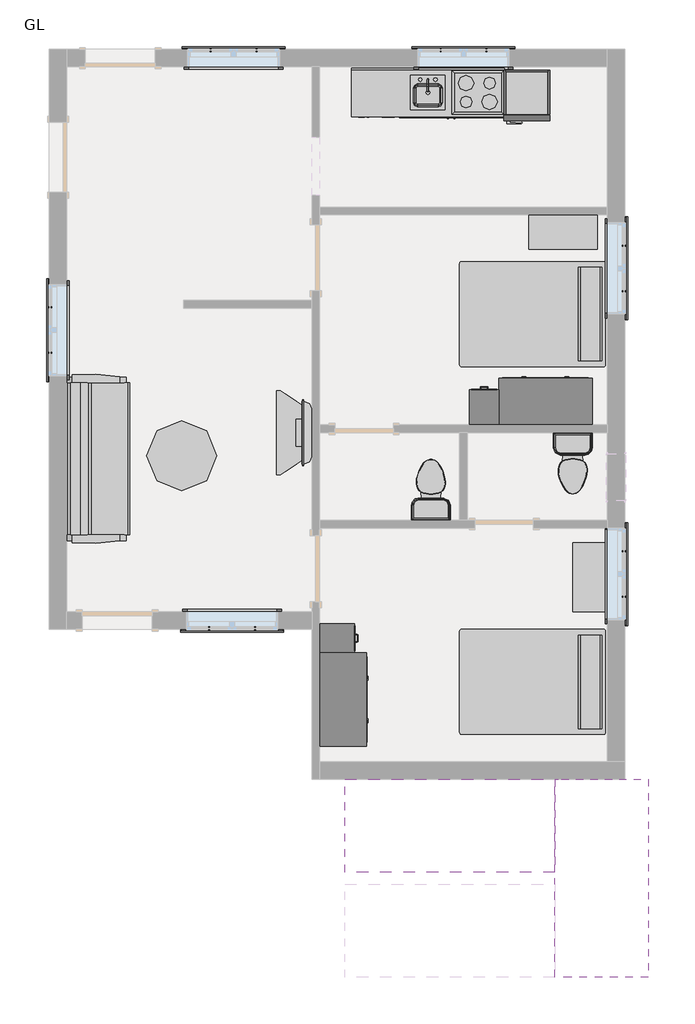
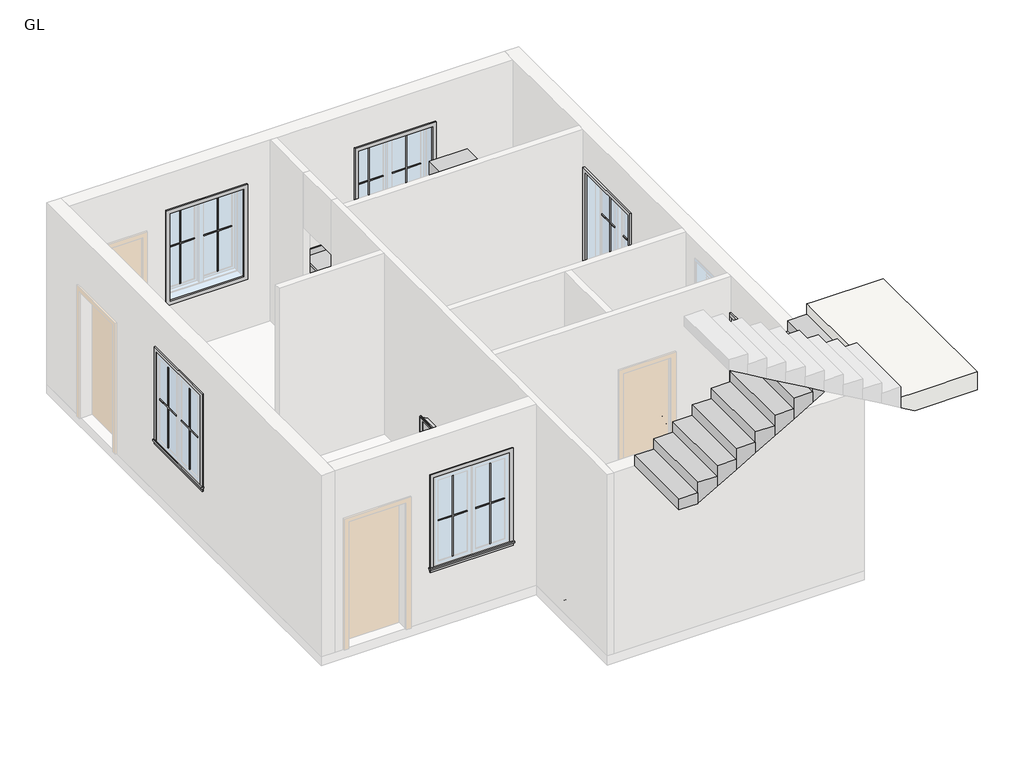
# One storey, part 2 of 2: 28 proxies, 13 furniture elements, 3 flow terminals, 1 slab, 1 stair flight.
"""IFC4 building model written with IfcOpenShell, lengths in millimetres."""

from ifc_helpers import new_model, si_unit, origin, place, context, project, spatial, faceted_brep, transform, mapped, element, save
from components import m_cook_top_4_unit2_0615_x_500mm_c91639ce, m_dishwasher_610_x_610_x_875mm_75336c20, m_kitchenette_medium_m_kitchenette_medium_71e50c56, m_muntin_pattern_2x2_m_muntin_pattern_2x2_d4676b39, m_muntin_pattern_2x2_m_muntin_pattern_2x2_dce6eb8c, m_refrigerator_600_x_660mm_0a899b9c, m_trim_window_exterior_flat_with_sill_a970d7bf, m_trim_window_interior_flat_picture_frame_5bf35ee4, m_sink_kitchen_island_450_x_450mm_f6c2c534, m_toilet_domestic_3d_m_toilet_domestic_3d_ba6479b0, m_toilet_domestic_3d_m_toilet_domestic_3d_1a010dbe, furniture_dc210597, furniture_0810mm_51289c3c, m_bed_standard_1372_x_1905mm_double_64e02cd7, m_cabinet_file_5_drawer_0380_x_0457mm_21dee09a, m_counter_top_w_sink_hole_600mm_depth_2c7d9717, m_dresser_1220_x_1830_x_0610mm_75a9f440, m_furniture_system_storage_cabinet_2_vertical_file_900_x_450_def3fd80, m_sofa_pensi_2134mm_538a523a, m_table_dining_round_0915mm_diameter_394c0b6d

model = new_model("IFC4")

# Units and contexts
model_context = context("Model", 3, world=origin())
ifc_project = project(units=[si_unit("LENGTHUNIT", "METRE", prefix="MILLI")], contexts=[model_context])

# Site, building, storey
site = spatial("IfcSite", under=ifc_project)
building = spatial("IfcBuilding", under=site)
storey = spatial("IfcBuildingStorey", under=building, Name="GL", Elevation=0.0)

# Proxies
placement = place(None, origin())
m_cook_top_4_unit2_0615_x_500mm_shape = m_cook_top_4_unit2_0615_x_500mm_c91639ce(model_context)
element("IfcBuildingElementProxy", 1, Name="M_Cook Top-4 Unit2 : 0615 x 500mm", ObjectType="M_Cook Top-4 Unit2 : 0615 x 500mm", at=placement, inside=storey, context=model_context, shape_type="MappedRepresentation", body=[
    mapped(m_cook_top_4_unit2_0615_x_500mm_shape, transform((1952.0701854, 4546.4851347, 15.0), x_axis=(-1.0, 0.0, 0.0), y_axis=(0.0, -1.0, 0.0), z_axis=(0.0, 0.0, 1.0))),
])
m_dishwasher_610_x_610_x_875mm_shape = m_dishwasher_610_x_610_x_875mm_75336c20(model_context)
element("IfcBuildingElementProxy", 2, Name="M_Dishwasher : 610 x 610 x 875mm", ObjectType="M_Dishwasher : 610 x 610 x 875mm", at=placement, inside=storey, context=model_context, shape_type="MappedRepresentation", body=[
    mapped(m_dishwasher_610_x_610_x_875mm_shape, transform((987.0876539, 4289.8355699, 0.0), x_axis=(-1.0, 0.0, 0.0), y_axis=(0.0, -1.0, 0.0), z_axis=(0.0, 0.0, 1.0))),
])
m_kitchenette_medium_m_kitchenette_medium_shape = m_kitchenette_medium_m_kitchenette_medium_71e50c56(model_context)
element("IfcBuildingElementProxy", 3, Name="M_Kitchenette - Medium : M_Kitchenette - Medium", ObjectType="M_Kitchenette - Medium : M_Kitchenette - Medium", at=placement, inside=storey, context=model_context, shape_type="MappedRepresentation", body=[
    mapped(m_kitchenette_medium_m_kitchenette_medium_shape, transform((1623.3078903, 4861.4851347, 0.0), x_axis=(-1.0, 0.0, 0.0), y_axis=(0.0, -1.0, 0.0), z_axis=(0.0, 0.0, 1.0))),
])
m_muntin_pattern_2x2_m_muntin_pattern_2x2_shape = m_muntin_pattern_2x2_m_muntin_pattern_2x2_d4676b39(model_context)
element("IfcBuildingElementProxy", 4, Name="M_Muntin Pattern_2x2 : M_Muntin Pattern_2x2", ObjectType="M_Muntin Pattern_2x2 : M_Muntin Pattern_2x2", at=placement, inside=storey, context=model_context, shape_type="MappedRepresentation", body=[
    mapped(m_muntin_pattern_2x2_m_muntin_pattern_2x2_shape, transform((1466.9330952, 5099.6101347, 969.85), x_axis=(1.0, 0.0, 0.0), y_axis=(0.0, 1.0, 0.0), z_axis=(0.0, 0.0, 1.0))),
])
element("IfcBuildingElementProxy", 5, Name="M_Muntin Pattern_2x2 : M_Muntin Pattern_2x2", ObjectType="M_Muntin Pattern_2x2 : M_Muntin Pattern_2x2", at=placement, inside=storey, context=model_context, shape_type="MappedRepresentation", body=[
    mapped(m_muntin_pattern_2x2_m_muntin_pattern_2x2_shape, transform((3864.0205952, 2548.5476347, 969.85), x_axis=(0.0, -1.0, 0.0), y_axis=(1.0, 0.0, 0.0), z_axis=(0.0, 0.0, 1.0))),
])
element("IfcBuildingElementProxy", 6, Name="M_Muntin Pattern_2x2 : M_Muntin Pattern_2x2", ObjectType="M_Muntin Pattern_2x2 : M_Muntin Pattern_2x2", at=placement, inside=storey, context=model_context, shape_type="MappedRepresentation", body=[
    mapped(m_muntin_pattern_2x2_m_muntin_pattern_2x2_shape, transform((3864.0205952, -1440.8523653, 969.85), x_axis=(0.0, -1.0, 0.0), y_axis=(1.0, 0.0, 0.0), z_axis=(0.0, 0.0, 1.0))),
])
element("IfcBuildingElementProxy", 7, Name="M_Muntin Pattern_2x2 : M_Muntin Pattern_2x2", ObjectType="M_Muntin Pattern_2x2 : M_Muntin Pattern_2x2", at=placement, inside=storey, context=model_context, shape_type="MappedRepresentation", body=[
    mapped(m_muntin_pattern_2x2_m_muntin_pattern_2x2_shape, transform((-960.1419048, -2450.5398653, 969.85), x_axis=(-1.0, 0.0, 0.0), y_axis=(0.0, -1.0, 0.0), z_axis=(0.0, 0.0, 1.0))),
])
element("IfcBuildingElementProxy", 8, Name="M_Muntin Pattern_2x2 : M_Muntin Pattern_2x2", ObjectType="M_Muntin Pattern_2x2 : M_Muntin Pattern_2x2", at=placement, inside=storey, context=model_context, shape_type="MappedRepresentation", body=[
    mapped(m_muntin_pattern_2x2_m_muntin_pattern_2x2_shape, transform((-3635.3294048, 1147.1226347, 969.85), x_axis=(0.0, 1.0, 0.0), y_axis=(-1.0, 0.0, 0.0), z_axis=(0.0, 0.0, 1.0))),
])
element("IfcBuildingElementProxy", 9, Name="M_Muntin Pattern_2x2 : M_Muntin Pattern_2x2", ObjectType="M_Muntin Pattern_2x2 : M_Muntin Pattern_2x2", at=placement, inside=storey, context=model_context, shape_type="MappedRepresentation", body=[
    mapped(m_muntin_pattern_2x2_m_muntin_pattern_2x2_shape, transform((-1536.9669048, 5099.6101347, 969.85), x_axis=(1.0, 0.0, 0.0), y_axis=(0.0, 1.0, 0.0), z_axis=(0.0, 0.0, 1.0))),
])
m_muntin_pattern_2x2_m_muntin_pattern_2x2_2_shape = m_muntin_pattern_2x2_m_muntin_pattern_2x2_dce6eb8c(model_context)
element("IfcBuildingElementProxy", 10, Name="M_Muntin Pattern_2x2 : M_Muntin Pattern_2x2", ObjectType="M_Muntin Pattern_2x2 : M_Muntin Pattern_2x2", at=placement, inside=storey, context=model_context, shape_type="MappedRepresentation", body=[
    mapped(m_muntin_pattern_2x2_m_muntin_pattern_2x2_2_shape, transform((2063.7580952, 5099.6101347, 969.85), x_axis=(-1.0, 0.0, 0.0), y_axis=(0.0, -1.0, 0.0), z_axis=(0.0, 0.0, 1.0))),
])
element("IfcBuildingElementProxy", 11, Name="M_Muntin Pattern_2x2 : M_Muntin Pattern_2x2", ObjectType="M_Muntin Pattern_2x2 : M_Muntin Pattern_2x2", at=placement, inside=storey, context=model_context, shape_type="MappedRepresentation", body=[
    mapped(m_muntin_pattern_2x2_m_muntin_pattern_2x2_2_shape, transform((3864.0205952, 1951.7226347, 969.85), x_axis=(0.0, 1.0, 0.0), y_axis=(-1.0, 0.0, 0.0), z_axis=(0.0, 0.0, 1.0))),
])
element("IfcBuildingElementProxy", 12, Name="M_Muntin Pattern_2x2 : M_Muntin Pattern_2x2", ObjectType="M_Muntin Pattern_2x2 : M_Muntin Pattern_2x2", at=placement, inside=storey, context=model_context, shape_type="MappedRepresentation", body=[
    mapped(m_muntin_pattern_2x2_m_muntin_pattern_2x2_2_shape, transform((3864.0205952, -2037.6773653, 969.85), x_axis=(0.0, 1.0, 0.0), y_axis=(-1.0, 0.0, 0.0), z_axis=(0.0, 0.0, 1.0))),
])
element("IfcBuildingElementProxy", 13, Name="M_Muntin Pattern_2x2 : M_Muntin Pattern_2x2", ObjectType="M_Muntin Pattern_2x2 : M_Muntin Pattern_2x2", at=placement, inside=storey, context=model_context, shape_type="MappedRepresentation", body=[
    mapped(m_muntin_pattern_2x2_m_muntin_pattern_2x2_2_shape, transform((-1556.9669048, -2450.5398653, 969.85), x_axis=(1.0, 0.0, 0.0), y_axis=(0.0, 1.0, 0.0), z_axis=(0.0, 0.0, 1.0))),
])
element("IfcBuildingElementProxy", 14, Name="M_Muntin Pattern_2x2 : M_Muntin Pattern_2x2", ObjectType="M_Muntin Pattern_2x2 : M_Muntin Pattern_2x2", at=placement, inside=storey, context=model_context, shape_type="MappedRepresentation", body=[
    mapped(m_muntin_pattern_2x2_m_muntin_pattern_2x2_2_shape, transform((-3635.3294048, 1743.9476347, 969.85), x_axis=(0.0, -1.0, 0.0), y_axis=(1.0, 0.0, 0.0), z_axis=(0.0, 0.0, 1.0))),
])
element("IfcBuildingElementProxy", 15, Name="M_Muntin Pattern_2x2 : M_Muntin Pattern_2x2", ObjectType="M_Muntin Pattern_2x2 : M_Muntin Pattern_2x2", at=placement, inside=storey, context=model_context, shape_type="MappedRepresentation", body=[
    mapped(m_muntin_pattern_2x2_m_muntin_pattern_2x2_2_shape, transform((-940.1419048, 5099.6101347, 969.85), x_axis=(-1.0, 0.0, 0.0), y_axis=(0.0, -1.0, 0.0), z_axis=(0.0, 0.0, 1.0))),
])
m_refrigerator_600_x_660mm_shape = m_refrigerator_600_x_660mm_0a899b9c(model_context)
element("IfcBuildingElementProxy", 16, Name="M_Refrigerator : 600 x 660mm", ObjectType="M_Refrigerator : 600 x 660mm", at=placement, inside=storey, context=model_context, shape_type="MappedRepresentation", body=[
    mapped(m_refrigerator_600_x_660mm_shape, transform((2541.7251841, 4544.3679413, 0.0), x_axis=(-1.0, 0.0, 0.0), y_axis=(0.0, -1.0, 0.0), z_axis=(0.0, 0.0, 1.0))),
])
m_trim_window_exterior_flat_with_sill_shape = m_trim_window_exterior_flat_with_sill_a970d7bf(model_context)
element("IfcBuildingElementProxy", 17, Name="M_Trim-Window-Exterior-Flat : with Sill", ObjectType="M_Trim-Window-Exterior-Flat : with Sill", at=placement, inside=storey, context=model_context, shape_type="MappedRepresentation", body=[
    mapped(m_trim_window_exterior_flat_with_sill_shape, transform((1765.3455952, 5109.1351347, 2400.0), x_axis=(-1.0, 0.0, 0.0), y_axis=(0.0, 0.0, 1.0), z_axis=(0.0, 1.0, 0.0))),
])
element("IfcBuildingElementProxy", 18, Name="M_Trim-Window-Exterior-Flat : with Sill", ObjectType="M_Trim-Window-Exterior-Flat : with Sill", at=placement, inside=storey, context=model_context, shape_type="MappedRepresentation", body=[
    mapped(m_trim_window_exterior_flat_with_sill_shape, transform((3873.5455952, 2250.1351347, 2400.0), x_axis=(0.0, 1.0, 0.0), y_axis=(0.0, 0.0, 1.0), z_axis=(1.0, 0.0, 0.0))),
])
element("IfcBuildingElementProxy", 19, Name="M_Trim-Window-Exterior-Flat : with Sill", ObjectType="M_Trim-Window-Exterior-Flat : with Sill", at=placement, inside=storey, context=model_context, shape_type="MappedRepresentation", body=[
    mapped(m_trim_window_exterior_flat_with_sill_shape, transform((3873.5455952, -1739.2648653, 2400.0), x_axis=(0.0, 1.0, 0.0), y_axis=(0.0, 0.0, 1.0), z_axis=(1.0, 0.0, 0.0))),
])
element("IfcBuildingElementProxy", 20, Name="M_Trim-Window-Exterior-Flat : with Sill", ObjectType="M_Trim-Window-Exterior-Flat : with Sill", at=placement, inside=storey, context=model_context, shape_type="MappedRepresentation", body=[
    mapped(m_trim_window_exterior_flat_with_sill_shape, transform((-1258.5544048, -2460.0648653, 2400.0), x_axis=(1.0, 0.0, 0.0), y_axis=(0.0, 0.0, 1.0), z_axis=(0.0, -1.0, 0.0))),
])
element("IfcBuildingElementProxy", 21, Name="M_Trim-Window-Exterior-Flat : with Sill", ObjectType="M_Trim-Window-Exterior-Flat : with Sill", at=placement, inside=storey, context=model_context, shape_type="MappedRepresentation", body=[
    mapped(m_trim_window_exterior_flat_with_sill_shape, transform((-3644.8544048, 1445.5351347, 2400.0), x_axis=(0.0, -1.0, 0.0), y_axis=(0.0, 0.0, 1.0), z_axis=(-1.0, 0.0, 0.0))),
])
element("IfcBuildingElementProxy", 22, Name="M_Trim-Window-Exterior-Flat : with Sill", ObjectType="M_Trim-Window-Exterior-Flat : with Sill", at=placement, inside=storey, context=model_context, shape_type="MappedRepresentation", body=[
    mapped(m_trim_window_exterior_flat_with_sill_shape, transform((-1238.5544048, 5109.1351347, 2400.0), x_axis=(-1.0, 0.0, 0.0), y_axis=(0.0, 0.0, 1.0), z_axis=(0.0, 1.0, 0.0))),
])
m_trim_window_interior_flat_picture_frame_shape = m_trim_window_interior_flat_picture_frame_5bf35ee4(model_context)
element("IfcBuildingElementProxy", 23, Name="M_Trim-Window-Interior-Flat : Picture Frame", ObjectType="M_Trim-Window-Interior-Flat : Picture Frame", at=placement, inside=storey, context=model_context, shape_type="MappedRepresentation", body=[
    mapped(m_trim_window_interior_flat_picture_frame_shape, transform((1765.3455952, 4880.5351347, 2400.0), x_axis=(1.0, 0.0, 0.0), y_axis=(0.0, 0.0, 1.0), z_axis=(0.0, -1.0, 0.0))),
])
element("IfcBuildingElementProxy", 24, Name="M_Trim-Window-Interior-Flat : Picture Frame", ObjectType="M_Trim-Window-Interior-Flat : Picture Frame", at=placement, inside=storey, context=model_context, shape_type="MappedRepresentation", body=[
    mapped(m_trim_window_interior_flat_picture_frame_shape, transform((3644.9455952, 2250.1351347, 2400.0), x_axis=(0.0, -1.0, 0.0), y_axis=(0.0, 0.0, 1.0), z_axis=(-1.0, 0.0, 0.0))),
])
element("IfcBuildingElementProxy", 25, Name="M_Trim-Window-Interior-Flat : Picture Frame", ObjectType="M_Trim-Window-Interior-Flat : Picture Frame", at=placement, inside=storey, context=model_context, shape_type="MappedRepresentation", body=[
    mapped(m_trim_window_interior_flat_picture_frame_shape, transform((3644.9455952, -1739.2648653, 2400.0), x_axis=(0.0, -1.0, 0.0), y_axis=(0.0, 0.0, 1.0), z_axis=(-1.0, 0.0, 0.0))),
])
element("IfcBuildingElementProxy", 26, Name="M_Trim-Window-Interior-Flat : Picture Frame", ObjectType="M_Trim-Window-Interior-Flat : Picture Frame", at=placement, inside=storey, context=model_context, shape_type="MappedRepresentation", body=[
    mapped(m_trim_window_interior_flat_picture_frame_shape, transform((-1258.5544048, -2231.4648653, 2400.0), x_axis=(-1.0, 0.0, 0.0), y_axis=(0.0, 0.0, 1.0), z_axis=(0.0, 1.0, 0.0))),
])
element("IfcBuildingElementProxy", 27, Name="M_Trim-Window-Interior-Flat : Picture Frame", ObjectType="M_Trim-Window-Interior-Flat : Picture Frame", at=placement, inside=storey, context=model_context, shape_type="MappedRepresentation", body=[
    mapped(m_trim_window_interior_flat_picture_frame_shape, transform((-3416.2544048, 1445.5351347, 2400.0), x_axis=(0.0, 1.0, 0.0), y_axis=(0.0, 0.0, 1.0), z_axis=(1.0, 0.0, 0.0))),
])
element("IfcBuildingElementProxy", 28, Name="M_Trim-Window-Interior-Flat : Picture Frame", ObjectType="M_Trim-Window-Interior-Flat : Picture Frame", at=placement, inside=storey, context=model_context, shape_type="MappedRepresentation", body=[
    mapped(m_trim_window_interior_flat_picture_frame_shape, transform((-1238.5544048, 4880.5351347, 2400.0), x_axis=(1.0, 0.0, 0.0), y_axis=(0.0, 0.0, 1.0), z_axis=(0.0, -1.0, 0.0))),
])

# Flow terminals
m_sink_kitchen_island_450_x_450mm_shape = m_sink_kitchen_island_450_x_450mm_f6c2c534(model_context)
element("IfcFlowTerminal", 29, ObjectType="M_Sink Kitchen-Island : 450 x 450mm", at=placement, inside=storey, context=model_context, shape_type="MappedRepresentation", body=[
    mapped(m_sink_kitchen_island_450_x_450mm_shape, transform((1315.2594259, 4546.0397336, 15.0), x_axis=(-1.0, 0.0, 0.0), y_axis=(0.0, -1.0, 0.0), z_axis=(0.0, 0.0, 1.0))),
])
m_toilet_domestic_3d_m_toilet_domestic_3d_shape = m_toilet_domestic_3d_m_toilet_domestic_3d_ba6479b0(model_context)
m_toilet_domestic_3d_m_toilet_domestic_3d_2_shape = m_toilet_domestic_3d_m_toilet_domestic_3d_1a010dbe(model_context)
element("IfcFlowTerminal", 30, ObjectType="M_Toilet-Domestic-3D : M_Toilet-Domestic-3D", at=placement, inside=storey, context=model_context, shape_type="MappedRepresentation", body=[
    mapped(m_toilet_domestic_3d_m_toilet_domestic_3d_shape, transform((3191.5495678, -389.3608926, 0.0), x_axis=(1.0, 0.0, 0.0), y_axis=(0.0, 1.0, 0.0), z_axis=(0.0, 0.0, 1.0))),
    mapped(m_toilet_domestic_3d_m_toilet_domestic_3d_2_shape, transform((3191.5495678, -389.3608926, 0.0), x_axis=(1.0, 0.0, 0.0), y_axis=(0.0, 1.0, 0.0), z_axis=(0.0, 0.0, 1.0))),
])
element("IfcFlowTerminal", 31, ObjectType="M_Toilet-Domestic-3D : M_Toilet-Domestic-3D", at=placement, inside=storey, context=model_context, shape_type="MappedRepresentation", body=[
    mapped(m_toilet_domestic_3d_m_toilet_domestic_3d_shape, transform((1339.1416225, -542.9688379, 0.0), x_axis=(-1.0, 0.0, 0.0), y_axis=(0.0, -1.0, 0.0), z_axis=(0.0, 0.0, 1.0))),
    mapped(m_toilet_domestic_3d_m_toilet_domestic_3d_2_shape, transform((1339.1416225, -542.9688379, 0.0), x_axis=(-1.0, 0.0, 0.0), y_axis=(0.0, -1.0, 0.0), z_axis=(0.0, 0.0, 1.0))),
])

# Furniture
furniture_shape = furniture_dc210597(model_context)
element("IfcFurniture", 32, at=placement, inside=storey, context=model_context, shape_type="MappedRepresentation", body=[
    mapped(furniture_shape, transform((-215.8544048, 230.5231368, 0.0), x_axis=(0.0, -1.0, 0.0), y_axis=(1.0, 0.0, 0.0), z_axis=(0.0, 0.0, 1.0))),
])
furniture_0810mm_shape = furniture_0810mm_51289c3c(model_context)
element("IfcFurniture", 33, ObjectType="0810mm", at=placement, inside=storey, context=model_context, shape_type="MappedRepresentation", body=[
    mapped(furniture_0810mm_shape, transform((-274.3930285, 101.3906206, 510.0), x_axis=(0.0, -1.0, 0.0), y_axis=(1.0, 0.0, 0.0), z_axis=(0.0, 0.0, 1.0))),
])
m_bed_standard_1372_x_1905mm_double_shape = m_bed_standard_1372_x_1905mm_double_64e02cd7(model_context)
element("IfcFurniture", 34, ObjectType="M_Bed-Standard : 1372 x 1905mm - Double", at=placement, inside=storey, context=model_context, shape_type="MappedRepresentation", body=[
    mapped(m_bed_standard_1372_x_1905mm_double_shape, transform((2712.6406772, -2874.5763407, 0.0), x_axis=(0.0, -1.0, 0.0), y_axis=(1.0, 0.0, 0.0), z_axis=(0.0, 0.0, 1.0))),
])
element("IfcFurniture", 35, ObjectType="M_Bed-Standard : 1372 x 1905mm - Double", at=placement, inside=storey, context=model_context, shape_type="MappedRepresentation", body=[
    mapped(m_bed_standard_1372_x_1905mm_double_shape, transform((2712.6406772, 1925.4236593, 0.0), x_axis=(0.0, -1.0, 0.0), y_axis=(1.0, 0.0, 0.0), z_axis=(0.0, 0.0, 1.0))),
])
m_cabinet_file_5_drawer_0380_x_0457mm_shape = m_cabinet_file_5_drawer_0380_x_0457mm_21dee09a(model_context)
element("IfcFurniture", 36, ObjectType="M_Cabinet-File 5 Drawer : 0380 x 0457mm", at=placement, inside=storey, context=model_context, shape_type="MappedRepresentation", body=[
    mapped(m_cabinet_file_5_drawer_0380_x_0457mm_shape, transform((-27.8887049, -2449.3684182, 0.0), x_axis=(0.0, 1.0, 0.0), y_axis=(-1.0, 0.0, 0.0), z_axis=(0.0, 0.0, 1.0))),
])
element("IfcFurniture", 37, ObjectType="M_Cabinet-File 5 Drawer : 0380 x 0457mm", at=placement, inside=storey, context=model_context, shape_type="MappedRepresentation", body=[
    mapped(m_cabinet_file_5_drawer_0380_x_0457mm_shape, transform((1907.0491482, 293.3008346, 0.0), x_axis=(-1.0, 0.0, 0.0), y_axis=(0.0, -1.0, 0.0), z_axis=(0.0, 0.0, 1.0))),
])
m_counter_top_w_sink_hole_600mm_depth_shape = m_counter_top_w_sink_hole_600mm_depth_2c7d9717(model_context)
element("IfcFurniture", 38, ObjectType="M_Counter Top w Sink Hole : 600mm Depth", at=placement, inside=storey, context=model_context, shape_type="MappedRepresentation", body=[
    mapped(m_counter_top_w_sink_hole_600mm_depth_shape, transform((1099.1078903, 4861.4851347, 15.0), x_axis=(-1.0, 0.0, 0.0), y_axis=(0.0, -1.0, 0.0), z_axis=(0.0, 0.0, 1.0))),
])
m_dresser_1220_x_1830_x_0610mm_shape = m_dresser_1220_x_1830_x_0610mm_75a9f440(model_context)
element("IfcFurniture", 39, ObjectType="M_Dresser : 1220 x 1830 x 0610mm", at=placement, inside=storey, context=model_context, shape_type="MappedRepresentation", body=[
    mapped(m_dresser_1220_x_1830_x_0610mm_shape, transform((2565.7523354, 148.7721806, 0.0), x_axis=(-1.0, 0.0, 0.0), y_axis=(0.0, -1.0, 0.0), z_axis=(0.0, 0.0, 1.0))),
])
element("IfcFurniture", 40, ObjectType="M_Dresser : 1220 x 1830 x 0610mm", at=placement, inside=storey, context=model_context, shape_type="MappedRepresentation", body=[
    mapped(m_dresser_1220_x_1830_x_0610mm_shape, transform((-172.4173589, -3108.0716054, 0.0), x_axis=(0.0, 1.0, 0.0), y_axis=(-1.0, 0.0, 0.0), z_axis=(0.0, 0.0, 1.0))),
])
m_furniture_system_storage_cabinet_2_vertical_file_900_x_450_shape = m_furniture_system_storage_cabinet_2_vertical_file_900_x_450_def3fd80(model_context)
element("IfcFurniture", 41, ObjectType="M_Furniture_System-Storage-Cabinet-2_Vertical_File : 900 x 450 x 650mm", at=placement, inside=storey, context=model_context, shape_type="MappedRepresentation", body=[
    mapped(m_furniture_system_storage_cabinet_2_vertical_file_900_x_450_shape, transform((3066.1455952, 2500.1351347, 0.0), x_axis=(1.0, 0.0, 0.0), y_axis=(0.0, 1.0, 0.0), z_axis=(0.0, 0.0, 1.0))),
])
element("IfcFurniture", 42, ObjectType="M_Furniture_System-Storage-Cabinet-2_Vertical_File : 900 x 450 x 650mm", at=placement, inside=storey, context=model_context, shape_type="MappedRepresentation", body=[
    mapped(m_furniture_system_storage_cabinet_2_vertical_file_900_x_450_shape, transform((3194.9455952, -1781.4648653, 0.0), x_axis=(0.0, -1.0, 0.0), y_axis=(1.0, 0.0, 0.0), z_axis=(0.0, 0.0, 1.0))),
])
m_sofa_pensi_2134mm_shape = m_sofa_pensi_2134mm_538a523a(model_context)
element("IfcFurniture", 43, ObjectType="M_Sofa-Pensi : 2134mm", at=placement, inside=storey, context=model_context, shape_type="MappedRepresentation", body=[
    mapped(m_sofa_pensi_2134mm_shape, transform((-2738.7445687, -514.3711153, 0.0), x_axis=(0.0, 1.0, 0.0), y_axis=(-1.0, 0.0, 0.0), z_axis=(0.0, 0.0, 1.0))),
])
m_table_dining_round_0915mm_diameter_shape = m_table_dining_round_0915mm_diameter_394c0b6d(model_context)
element("IfcFurniture", 44, ObjectType="M_Table-Dining Round : 0915mm Diameter", at=placement, inside=storey, context=model_context, shape_type="MappedRepresentation", body=[
    mapped(m_table_dining_round_0915mm_diameter_shape, transform((-2019.536372, -9.7861767, 0.0), x_axis=(1.0, 0.0, 0.0), y_axis=(0.0, 1.0, 0.0), z_axis=(0.0, 0.0, 1.0))),
])

# Slab
element("IfcSlab", 45, ObjectType="300mm Thickness", at=placement, inside=storey, context=model_context, shape_type="Brep", body=[
    faceted_brep([(2959.1455952, -4415.8648653, 4812.6315789), (2959.1455952, -5635.0648653, 4812.6315789), (2959.1455952, -5787.4648653, 4812.6315789), (2959.1455952, -7006.6648653, 4812.6315789), (3177.9478897, -7006.6648653, 4812.6315789), (4178.3455952, -7006.6648653, 4812.6315789), (4178.3455952, -4415.8648653, 4812.6315789), (3045.1433006, -4415.8648653, 4812.6315789), (2959.1455952, -4415.8648653, 4636.1684211), (2959.1455952, -4415.8648653, 4462.8434337), (2959.1455952, -5635.0648653, 4462.8434337), (2959.1455952, -5635.0648653, 4512.6315789), (2959.1455952, -5787.4648653, 4512.6315789), (2959.1455952, -5787.4648653, 4639.3065916), (2959.1455952, -7006.6648653, 4639.3065916), (3177.9478897, -7006.6648653, 4512.6315789), (4178.3455952, -7006.6648653, 4512.6315789), (4178.3455952, -4415.8648653, 4512.6315789), (3045.1433006, -4415.8648653, 4512.6315789), (3177.9478897, -5787.4648653, 4512.6315789), (3045.1433006, -5635.0648653, 4512.6315789)], [[[0, 1, 2, 3, 4, 5, 6, 7]], [[1, 0, 8, 9, 10, 11]], [[2, 1, 11, 12, 13]], [[3, 2, 13, 14]], [[3, 14, 15, 16, 5, 4]], [[6, 5, 16, 17]], [[9, 8, 0, 7, 6, 17, 18]], [[19, 12, 11, 20, 18, 17, 16, 15]], [[12, 19, 13]], [[18, 20, 10, 9]], [[20, 11, 10]], [[19, 15, 14, 13]]]),
])

# Stair flight
element("IfcStairFlight", 46, ObjectType="150mm Depth", at=placement, inside=storey, context=model_context, shape_type="Brep", body=[
    faceted_brep([(520.7455952, -4415.8648653, 3224.4631579), (215.9455952, -4415.8648653, 3224.4631579), (215.9455952, -5635.0648653, 3224.4631579), (520.7455952, -5635.0648653, 3224.4631579), (520.7455952, -4415.8648653, 3051.1381705), (515.3251188, -4415.8648653, 3048.0), (215.9455952, -4415.8648653, 3048.0), (215.9455952, -5635.0648653, 3048.0), (515.3251188, -5635.0648653, 3048.0), (520.7455952, -5635.0648653, 3051.1381705), (825.5455952, -4415.8648653, 3400.9263158), (520.7455952, -4415.8648653, 3400.9263158), (520.7455952, -5635.0648653, 3400.9263158), (825.5455952, -5635.0648653, 3400.9263158), (825.5455952, -4415.8648653, 3227.6013284), (825.5455952, -5635.0648653, 3227.6013284), (1130.3455952, -4415.8648653, 3577.3894737), (825.5455952, -4415.8648653, 3577.3894737), (825.5455952, -5635.0648653, 3577.3894737), (1130.3455952, -5635.0648653, 3577.3894737), (1130.3455952, -4415.8648653, 3404.0644863), (1130.3455952, -5635.0648653, 3404.0644863), (1435.1455952, -4415.8648653, 3753.8526316), (1130.3455952, -4415.8648653, 3753.8526316), (1130.3455952, -5635.0648653, 3753.8526316), (1435.1455952, -5635.0648653, 3753.8526316), (1435.1455952, -4415.8648653, 3580.5276442), (1435.1455952, -5635.0648653, 3580.5276442), (1739.9455952, -4415.8648653, 3930.3157895), (1435.1455952, -4415.8648653, 3930.3157895), (1435.1455952, -5635.0648653, 3930.3157895), (1739.9455952, -5635.0648653, 3930.3157895), (1739.9455952, -4415.8648653, 3756.9908021), (1739.9455952, -5635.0648653, 3756.9908021), (2044.7455952, -4415.8648653, 4106.7789474), (1739.9455952, -4415.8648653, 4106.7789474), (1739.9455952, -5635.0648653, 4106.7789474), (2044.7455952, -5635.0648653, 4106.7789474), (2044.7455952, -4415.8648653, 3933.45396), (2044.7455952, -5635.0648653, 3933.45396), (2349.5455952, -4415.8648653, 4283.2421053), (2044.7455952, -4415.8648653, 4283.2421053), (2044.7455952, -5635.0648653, 4283.2421053), (2349.5455952, -5635.0648653, 4283.2421053), (2349.5455952, -4415.8648653, 4109.9171179), (2349.5455952, -5635.0648653, 4109.9171179), (2654.3455952, -4415.8648653, 4459.7052632), (2349.5455952, -4415.8648653, 4459.7052632), (2349.5455952, -5635.0648653, 4459.7052632), (2654.3455952, -5635.0648653, 4459.7052632), (2654.3455952, -4415.8648653, 4286.3802758), (2654.3455952, -5635.0648653, 4286.3802758), (2959.1455952, -4415.8648653, 4636.1684211), (2654.3455952, -4415.8648653, 4636.1684211), (2654.3455952, -5635.0648653, 4636.1684211), (2959.1455952, -5635.0648653, 4636.1684211), (2959.1455952, -4415.8648653, 4462.8434337), (2959.1455952, -5635.0648653, 4462.8434337), (2959.1455952, -5635.0648653, 4512.6315789)], [[[0, 1, 2, 3]], [[1, 0, 4, 5, 6]], [[2, 1, 6, 7]], [[3, 2, 7, 8, 9]], [[10, 11, 12, 13]], [[11, 10, 14, 4, 0]], [[0, 3, 12, 11]], [[13, 12, 3, 9, 15]], [[16, 17, 18, 19]], [[17, 16, 20, 14, 10]], [[10, 13, 18, 17]], [[19, 18, 13, 15, 21]], [[22, 23, 24, 25]], [[23, 22, 26, 20, 16]], [[16, 19, 24, 23]], [[25, 24, 19, 21, 27]], [[28, 29, 30, 31]], [[29, 28, 32, 26, 22]], [[22, 25, 30, 29]], [[31, 30, 25, 27, 33]], [[34, 35, 36, 37]], [[35, 34, 38, 32, 28]], [[28, 31, 36, 35]], [[37, 36, 31, 33, 39]], [[40, 41, 42, 43]], [[41, 40, 44, 38, 34]], [[34, 37, 42, 41]], [[43, 42, 37, 39, 45]], [[46, 47, 48, 49]], [[47, 46, 50, 44, 40]], [[40, 43, 48, 47]], [[49, 48, 43, 45, 51]], [[52, 53, 54, 55]], [[53, 52, 56, 50, 46]], [[46, 49, 54, 53]], [[55, 54, 49, 51, 57, 58]], [[52, 55, 58, 57, 56]], [[7, 6, 5, 8]], [[8, 5, 4, 14, 20, 26, 32, 38, 44, 50, 56, 57, 51, 45, 39, 33, 27, 21, 15, 9]]]),
])

save(model, "model.ifc")

# Revit data of these elements
# Type "M_Cook Top-4 Unit2 : 0615 x 500mm"
#   Depth = 1.64042 ft
#   Width = 2.017717 ft
#   Burner Material = Steel, Chrome Plated
#   Cooktop Material = Steel, Polished
#   Default Elevation = 0
#   Assembly Code = ""
# Type "M_Dishwasher : 610 x 610 x 875mm"
#   Label = "DW"
#   Depth = 2.001312 ft
#   Height = 2.870735 ft
#   Width = 2.001312 ft
#   Dishwasher Material = Steel, Paint Finish, Ivory, Glossy
#   Panel Face Material = Plastic, Opaque Black
#   Default Elevation = 0
# Type "M_Kitchenette - Medium : M_Kitchenette - Medium"
#   Sink Opening Depth = 1.148294 ft
#   Sink Location To Wall = 0.492126 ft
#   Sink Location = 3.28084 ft
#   Counter Thickness = 0.131234 ft
#   Counter Length = 6.56168 ft
#   Cabinet Width = 4.560367 ft
#   Cabinet Height = 2.870735 ft
#   Cabinet Depth = 2.066929 ft
#   Toe Depth = 0.114829 ft
#   Toe Height = 0.328084 ft
#   Cabinet Material = Cabinets
#   Door/Drawer Material = Cabinets
#   Handle Material = Cabinets - Handles
#   Default Elevation = 0
# Type "M_Muntin Pattern_2x2 : M_Muntin Pattern_2x2"
#   Width [instance default] = 3.937008 ft
#   Thickness = 0.041667 ft
#   Height [instance default] = 3.937008 ft
#   Distance = 0.0625 ft
#   Interior Material [instance default] = none
#   Exterior Material [instance default] = none
#   Default Elevation = 0
# Type "M_Refrigerator : 600 x 660mm"
#   Label = "REF."
#   Depth = 2.165354 ft
#   Height = 6.003937 ft
#   Width = 1.968504 ft
#   Material = Steel, Paint Finish, Ivory, Matte
#   Description = (empty or 0)
#   Default Elevation = 0
# Type "M_Trim-Window-Exterior-Flat : with Sill"
#   Trim Width = 0.19685 ft
#   Trim Thickness_Picture Frame = 0.098425 ft
#   Trim Thickness_with Sill = 0.0625 ft
#   Sill Thickness = 0.098425 ft
#   Opening Width [instance default] = 1.968504 ft
#   Opening Height [instance default] = 2.952756 ft
#   Default Elevation = 3.937008 ft
#   Sill = yes
#   Picture Frame = no
#   Trim Material [instance default] = none
# Type "M_Trim-Window-Interior-Flat : Picture Frame"
#   Trim Thickness_Picture Frame = 0.098425 ft
#   Trim Width = 0.19685 ft
#   Trim Thickness_with Sill = 0.065617 ft
#   Sill Thickness = 0.098425 ft
#   Opening Width [instance default] = 1.968504 ft
#   Opening Height [instance default] = 2.952756 ft
#   Default Elevation = 3.937008 ft
#   Sill = no
#   Picture Frame = yes
#   Trim Material [instance default] = none
# Type "M_Sink Kitchen-Island : 450 x 450mm"
#   Counter Height [instance default] = 2.952756 ft
#   Depth = 1.476378 ft
#   Width = 1.476378 ft
#   Fixture Material = Steel, Polished
#   Sink Material = Steel, Polished
#   Default Elevation = 0
# Type "M_Toilet-Domestic-3D : M_Toilet-Domestic-3D"
#   Bowl/Basin Material = Porcelain, Linen
#   Seat Material = Laminate, Linen, Matte
#   Default Elevation = 0
# Type
#   Depth = 1.509186 ft
#   Width = 3.608924 ft
#   Height = 1.64042 ft
#   Finish = Melamine - Gray
#   Default Elevation = 0
# Type "0810mm"
#   SinAng = 0.001609 ft
#   L = 2.316144 ft
#   H = 1.30295 ft
#   Thickness = 0.360892 ft
#   Diagonal = 2.65748 ft
#   CosAng = 0.002859 ft
#   Stand [instance default] = yes
#   Default Elevation = 0
# Type "M_Bed-Standard : 1372 x 1905mm - Double"
#   Length = 6.25 ft
#   Width = 4.501312 ft
#   Leg Material = Steel, Chrome Plated
#   Mattress Material = Linen, White
#   Default Elevation = 0
# Type "M_Cabinet-File 5 Drawer : 0380 x 0457mm"
#   Depth = 1.499344 ft
#   Height = 5.003281 ft
#   Width = 1.246719 ft
#   Cabinet Material = Steel, Paint Finish, Ivory, Glossy
#   Handle Material = Steel, Chrome Plated
#   Default Elevation = 0
# Type "M_Counter Top w Sink Hole : 600mm Depth"
#   Counter Thickness = 0.131234 ft
#   Depth [instance default] = 2.050525 ft
#   Height = 2.952756 ft
#   Length [instance default] = 8.2021 ft
#   Sink Location [instance default] = 3.937008 ft
#   Sink Location To Wall [instance default] = 0.328084 ft
#   Sink Opening Depth [instance default] = 1.240157 ft
#   Sink Opening Width [instance default] = 1.925853 ft
#   Counter Top Material = none
#   Default Elevation = 0
# Type "M_Dresser : 1220 x 1830 x 0610mm"
#   Depth = 2.001312 ft
#   Height = 6.003937 ft
#   Width = 4.002625 ft
#   Dresser Material = Laminate - Ivory, Glossy
#   Drawer Material = Laminate, Ivory, Matte
#   Knob Material = Cherry
#   Default Elevation = 0
# Type "M_Furniture_System-Storage-Cabinet-2_Vertical_File : 900 x 450 x 650mm"
#   Type Comments = "900 x 450 x 650mm Double Vertical File Cabinet"
#   Width = 2.952756 ft
#   Height = 2.132546 ft
#   Depth = 1.476378 ft
#   Show Solid [instance default] = yes
#   Show Dashed [instance default] = no
#   Drawer Finish [instance default] = Metal - Paint - Beige
#   Cabinet Material [instance default] = Metal - Paint - Beige
#   Model = ""
#   Manufacturer = ""
#   Description = (empty or 0)
#   Default Elevation = 0
# Type "M_Sofa-Pensi : 2134mm"
#   Length = 7.001312 ft
#   Sofa Material = Linen, Beige
#   Frame Material = Steel, Chrome Plated
#   Default Elevation = 0
# Type "M_Table-Dining Round : 0915mm Diameter"
#   Diameter = 3.001969 ft
#   Height = 2.5 ft
#   Base Material = Pine
#   Top Material = Laminate, Linen, Matte
#   Default Elevation = 0
# Element 1 (IfcBuildingElementProxy, "M_Cook Top-4 Unit2 : 0615 x 500mm")
#   Phase Created = New Construction
#   Materials on its faces: "Steel, Polished", "Steel, Chrome Plated"
# Element 2 (IfcBuildingElementProxy, "M_Dishwasher : 610 x 610 x 875mm")
#   Phase Created = New Construction
#   Materials on its faces: "Steel, Paint Finish, Ivory, Glossy", "Plastic, Opaque Black"
# Element 3 (IfcBuildingElementProxy, "M_Kitchenette - Medium : M_Kitchenette - Medium")
#   Phase Created = New Construction
#   Materials on its faces: "Cabinets", "Cabinets - Handles"
# Elements 4, 5, 6, 7, 8, 9, 10, 11, 12, 13, 14, 15 (IfcBuildingElementProxy, "M_Muntin Pattern_2x2 : M_Muntin Pattern_2x2")
#   Width = 1.520587 ft
#   Height = 4.462927 ft
#   Interior Material = Wood - Stained
#   Exterior Material = Clad - White
#   Phase Created = New Construction
#   Materials on its faces: "Clad - White", "Wood - Stained"
# Element 16 (IfcBuildingElementProxy, "M_Refrigerator : 600 x 660mm")
#   Phase Created = New Construction
#   Materials on its faces: "Steel, Paint Finish, Ivory, Matte", "Steel, Chrome Plated"
# Elements 17, 18, 19, 20, 21, 22 (IfcBuildingElementProxy, "M_Trim-Window-Exterior-Flat : with Sill")
#   Opening Width = 3.937008 ft
#   Opening Height = 4.92126 ft
#   Trim Material = Clad - White
#   Phase Created = New Construction
#   Materials on its faces: "Clad - White"
# Elements 23, 24, 25, 26, 27, 28 (IfcBuildingElementProxy, "M_Trim-Window-Interior-Flat : Picture Frame")
#   Opening Width = 3.937008 ft
#   Opening Height = 4.92126 ft
#   Trim Material = Wood - Stained
#   Phase Created = New Construction
#   Materials on its faces: "Wood - Stained"
# Element 29 (IfcFlowTerminal, "M_Sink Kitchen-Island : 450 x 450mm")
#   Mark = "3"
#   Counter Height = 2.952756 ft
#   Phase Created = New Construction
#   Materials on its faces: "Steel, Polished"
# Element 30 (IfcFlowTerminal, "M_Toilet-Domestic-3D : M_Toilet-Domestic-3D")
#   Mark = "4"
#   Phase Created = New Construction
#   Materials on its faces: "Porcelain, Linen", "Laminate, Linen, Matte"
# Element 31 (IfcFlowTerminal, "M_Toilet-Domestic-3D : M_Toilet-Domestic-3D")
#   Mark = "5"
#   Phase Created = New Construction
#   Materials on its faces: "Porcelain, Linen", "Laminate, Linen, Matte"
# Element 32 (IfcFurniture)
#   Phase Created = New Construction
#   Materials on its faces: "Melamine - Gray", "Glass - Shelves"
# Element 33 (IfcFurniture, "0810mm")
#   Stand = yes
#   Phase Created = New Construction
#   Materials on its faces: "TV - Black", "TV - Glass", "TV - Screen"
# Elements 34, 35 (IfcFurniture, "M_Bed-Standard : 1372 x 1905mm - Double")
#   Phase Created = New Construction
#   Materials on its faces: "Linen, White", "Steel, Chrome Plated"
# Elements 36, 37 (IfcFurniture, "M_Cabinet-File 5 Drawer : 0380 x 0457mm")
#   Phase Created = New Construction
#   Materials on its faces: "Steel, Chrome Plated", "Steel, Paint Finish, Ivory, Glossy"
# Element 38 (IfcFurniture, "M_Counter Top w Sink Hole : 600mm Depth")
#   Sink Opening Width = 1.312336 ft
#   Sink Opening Depth = 1.148294 ft
#   Sink Location To Wall = 0.492126 ft
#   Sink Location = 3.28084 ft
#   Length = 6.56168 ft
#   Depth = 2.066929 ft
#   Phase Created = New Construction
#   Materials on its faces: "Counter Top"
# Elements 39, 40 (IfcFurniture, "M_Dresser : 1220 x 1830 x 0610mm")
#   Phase Created = New Construction
#   Materials on its faces: "Laminate, Ivory, Matte", "Cherry", "Laminate - Ivory, Glossy"
# Elements 41, 42 (IfcFurniture, "M_Furniture_System-Storage-Cabinet-2_Vertical_File : 900 x 450 x 650mm")
#   Show Solid = yes
#   Show Dashed = no
#   Drawer Finish = Metal - Paint - Beige
#   Cabinet Material = Metal - Paint - Beige
#   Phase Created = New Construction
#   Materials on its faces: "Metal - Paint - Beige"
# Element 43 (IfcFurniture, "M_Sofa-Pensi : 2134mm")
#   Phase Created = New Construction
#   Materials on its faces: "Linen, Beige", "Steel, Chrome Plated"
# Element 44 (IfcFurniture, "M_Table-Dining Round : 0915mm Diameter")
#   Phase Created = New Construction
#   Materials on its faces: "Pine", "Laminate, Linen, Matte"
# Element 45 (IfcSlab, "300mm Thickness")
#   Phase Created = New Construction
#   Materials on its faces: "Concrete, Cast In Situ"
# Element 46 (IfcStairFlight, "150mm Depth")
#   Phase Created = New Construction
#   Materials on its faces: "Concrete, Cast In Situ"
# Materials
#   "Steel, Chrome Plated": class "Metal", colour RGB 17 17 17, transparency 0, Description = "Chromiuim plated steel", Cost = 0
#   "Steel, Polished": class "Metal", colour RGB 57 57 57, transparency 0, Description = "Polished steel", Cost = 0
#   "Steel, Paint Finish, Ivory, Glossy": class "Metal", colour RGB 247 247 239, transparency 0, Description = "Steel, paint finish, ivory, glossy", Cost = 0
#   "Plastic, Opaque Black": class "Plastic", colour RGB 0 0 0, transparency 0.7, Description = "Plastic, generic, opaque black", Cost = 0
#   "Cabinets": colour RGB 249 249 249, transparency 0
#   "Cabinets - Handles": class "Metal", colour RGB 57 57 57, transparency 0
#   "Steel, Paint Finish, Ivory, Matte": class "Metal", colour RGB 247 247 239, transparency 0, Description = "Steel, paint finish, ivory, matte", Cost = 0
#   "Porcelain, Linen": class "Ceramic", colour RGB 249 239 230, transparency 0, Description = "Porcelain, linen", Cost = 0
#   "Laminate, Linen, Matte": class "Plastic", colour RGB 249 239 230, transparency 0, Description = "Plastic Laminate - Linen, Matte", Cost = 0
#   "Melamine - Gray": class "Wood", colour RGB 49 49 49, transparency 0
#   "Linen, White": class "Textile", colour RGB 247 247 239, transparency 0, Description = "Linen, white", Cost = 0
#   "Laminate - Ivory, Glossy": colour RGB 247 247 239, transparency 0
#   "Laminate, Ivory, Matte": class "Plastic", colour RGB 247 247 239, transparency 0, Description = "Plastic Laminate - Ivory, Matte", Cost = 0
#   "Cherry": class "Wood", colour RGB 226 177 128, transparency 0, Description = "Prunus Serotina", Cost = 0
#   "Metal - Paint - Beige": class "Metal", colour RGB 247 225 182, transparency 0
#   "Linen, Beige": class "Textile", colour RGB 249 239 230, transparency 0, Description = "Linen, beige", Cost = 0
#   "Pine": class "Wood", colour RGB 223 192 134, transparency 0, Description = "Pinus Echinata", Cost = 0
#   "Clad - White": class "Wood", colour RGB 242 242 238, transparency 0, Cost = 0
#   "Wood - Stained": class "Wood", colour RGB 224 178 126, transparency 0, Cost = 0
#   "Glass - Shelves": class "Glass", colour RGB 167 167 167, transparency 0.9
#   "TV - Black": colour RGB 49 49 49, transparency 0
#   "TV - Glass": colour RGB 157 157 157, transparency 0.9
#   "TV - Screen": colour RGB 0 0 0, transparency 0
#   "Counter Top": class "Wood", colour RGB 226 177 128, transparency 0
#   "Concrete, Cast In Situ": class "Concrete", colour RGB 192 192 192, transparency 0, Description = "physical material", Cost = 0
